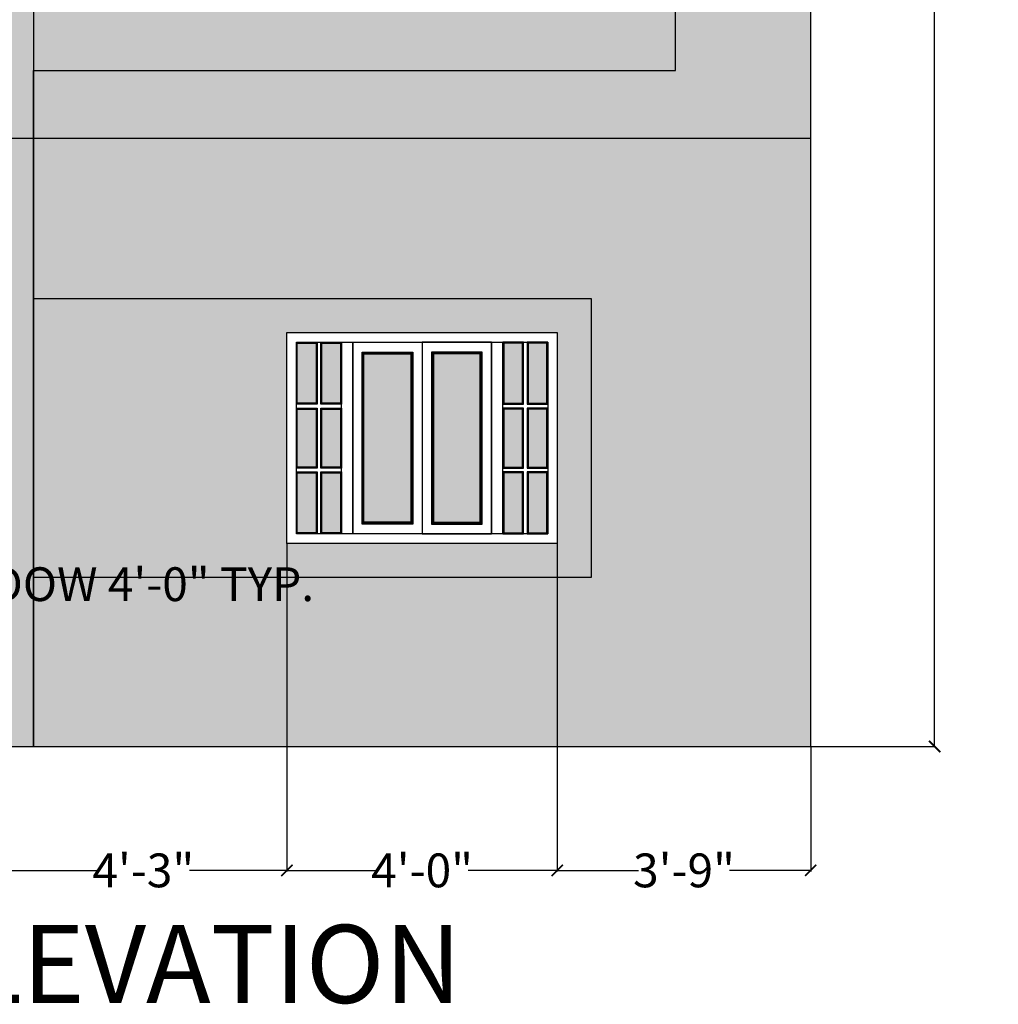
# Model space of a CAD drawing. Units: inches. Extents: x 528 to 2620, y -1066 to 798.
# Tile 39 of 41: x 2446 to 2620, y -1066 to -891. Entities that reach past the tile are written whole.
import ezdxf

# ---------------------------------------------------------------- set-up
doc = ezdxf.new("R2010")
doc.units = ezdxf.units.IN
doc.header["$MEASUREMENT"] = 0
for name, color, linetype, lineweight in [('A-ANNO-DIMS', 2, 'Continuous', 18), ('A-ANNO-TEXT', 7, 'Continuous', 25), ('A-ELEV', 7, 'Continuous', 25), ('A-ELEV-PATT', 8, 'Continuous', 13)]:
    doc.layers.add(name, color=color, linetype=linetype, lineweight=lineweight)
doc.styles.get("Standard").update_dxf_attribs({"font": 'arial.ttf'})
doc.dimstyles.get("Standard").update_dxf_attribs({"dimtxt": 6, "dimasz": 2, "dimexe": 0.18, "dimexo": 0.0625, "dimgap": 0.09, "dimtad": 0, "dimtih": 1, "dimtoh": 1, "dimdec": 1, "dimzin": 0, "dimdsep": 46, "dimlunit": 3, "dimtxsty": 'Standard', "dimblk": 'ARCHTICK', "dimcen": 0.09, "dimadec": 0, "dimazin": 0, "dimtfac": 1, "dimtdec": 1, "dimtofl": 0, "dimtmove": 0, "dimatfit": 3, "dimfxl": 1, "dimtolj": 1, "dimtzin": 0, "dimarcsym": 0})

# ---------------------------------------------------------------- blocks, each defined once
blk = doc.blocks.new('ww')
at = {"color": 0, "linetype": 'ByBlock'}
for p, q in [((30.67, -16.13), (126.65, -16.13)), ((30.67, -91.08), (30.67, -16.13)), ((126.65, -16.13), (126.65, -91.08)), ((34.01, -19.6), (123.32, -19.6)), ((34.01, -87.61), (34.01, -19.6)), ((34.01, -19.6), (49.87, -19.6)), ((34.01, -87.61), (34.01, -19.6)), ((50.03, -87.61), (50.03, -19.6)), ((54.03, -19.6), (54.03, -87.61)), ((103.29, -19.6), (103.29, -87.61)), ((107.29, -87.61), (107.29, -19.6)), ((123.32, -19.6), (123.32, -87.61)), ((123.32, -87.61), (34.01, -87.61)), ((126.65, -91.08), (30.67, -91.08))]:
    blk.add_line(p, q, dxfattribs=at)
at = {"color": 0, "linetype": 'ByBlock', "ltscale": 25}
for p, q in [((34.01, -41.58), (34.01, -19.6)), ((34.01, -19.6), (41.35, -19.6)), ((34.34, -41.23), (34.34, -19.95)), ((34.34, -19.95), (41.02, -19.95)), ((41.02, -19.95), (41.02, -41.23)), ((41.35, -19.6), (41.35, -41.58)), ((42.69, -41.58), (42.69, -19.6)), ((42.69, -19.6), (50.03, -19.6)), ((43.02, -41.23), (43.02, -19.95)), ((43.02, -19.95), (49.7, -19.95)), ((49.7, -19.95), (49.7, -41.23)), ((50.03, -19.6), (50.03, -41.58)), ((54.03, -87.61), (54.03, -19.6)), ((54.03, -19.6), (78.66, -19.6)), ((103.29, -19.6), (78.66, -19.6)), ((78.66, -19.6), (78.66, -87.61)), ((78.66, -19.6), (78.66, -87.61)), ((103.29, -87.61), (103.29, -19.6)), ((107.29, -19.6), (107.29, -41.58)), ((114.63, -19.6), (107.29, -19.6)), ((107.62, -19.95), (107.62, -41.23)), ((114.3, -19.95), (107.62, -19.95)), ((114.3, -41.23), (114.3, -19.95)), ((114.63, -41.58), (114.63, -19.6)), ((115.97, -19.6), (115.97, -41.58)), ((123.32, -19.6), (115.97, -19.6)), ((116.3, -19.95), (116.3, -41.23)), ((122.98, -19.95), (116.3, -19.95)), ((122.98, -41.23), (122.98, -19.95)), ((123.32, -41.58), (123.32, -19.6)), ((57.37, -84.14), (57.37, -23.07)), ((57.37, -23.07), (75.33, -23.07)), ((57.7, -83.8), (57.7, -23.42)), ((57.7, -23.42), (74.99, -23.42)), ((58.03, -83.45), (58.03, -23.77)), ((58.03, -23.77), (74.66, -23.77)), ((74.66, -23.77), (74.66, -83.45)), ((74.99, -23.42), (74.99, -83.8)), ((75.33, -23.07), (75.33, -84.14)), ((99.96, -23.07), (81.99, -23.07)), ((81.99, -23.07), (81.99, -84.14)), ((99.62, -23.42), (82.33, -23.42)), ((82.33, -23.42), (82.33, -83.8)), ((99.29, -23.77), (82.66, -23.77)), ((82.66, -23.77), (82.66, -83.45)), ((99.29, -83.45), (99.29, -23.77)), ((99.62, -83.8), (99.62, -23.42)), ((99.96, -84.14), (99.96, -23.07)), ((41.35, -41.58), (34.01, -41.58)), ((41.02, -41.23), (34.34, -41.23)), ((50.03, -41.58), (42.69, -41.58)), ((49.7, -41.23), (43.02, -41.23)), ((107.29, -41.58), (114.63, -41.58)), ((107.62, -41.23), (114.3, -41.23)), ((115.97, -41.58), (123.32, -41.58)), ((116.3, -41.23), (122.98, -41.23)), ((34.01, -64.25), (34.01, -42.97)), ((34.01, -42.97), (41.35, -42.97)), ((34.34, -63.9), (34.34, -43.31)), ((34.34, -43.31), (41.02, -43.31)), ((41.02, -43.31), (41.02, -63.9)), ((41.35, -42.97), (41.35, -64.25)), ((42.69, -64.25), (42.69, -42.97)), ((42.69, -42.97), (50.03, -42.97)), ((43.02, -63.9), (43.02, -43.31)), ((43.02, -43.31), (49.7, -43.31)), ((49.7, -43.31), (49.7, -63.9)), ((50.03, -42.97), (50.03, -64.25)), ((107.29, -42.97), (107.29, -64.25)), ((114.63, -42.97), (107.29, -42.97)), ((107.62, -43.31), (107.62, -63.9)), ((114.3, -43.31), (107.62, -43.31)), ((114.3, -63.9), (114.3, -43.31)), ((114.63, -64.25), (114.63, -42.97)), ((115.97, -42.97), (115.97, -64.25)), ((123.32, -42.97), (115.97, -42.97)), ((116.3, -43.31), (116.3, -63.9)), ((122.98, -43.31), (116.3, -43.31)), ((122.98, -63.9), (122.98, -43.31)), ((123.32, -64.25), (123.32, -42.97)), ((41.35, -64.25), (34.01, -64.25)), ((34.01, -87.61), (34.01, -65.64)), ((34.01, -65.64), (41.35, -65.64)), ((41.02, -63.9), (34.34, -63.9)), ((34.34, -87.27), (34.34, -65.98)), ((34.34, -65.98), (41.02, -65.98)), ((41.02, -65.98), (41.02, -87.27)), ((41.35, -65.64), (41.35, -87.61)), ((50.03, -64.25), (42.69, -64.25)), ((42.69, -87.61), (42.69, -65.64)), ((42.69, -65.64), (50.03, -65.64)), ((49.7, -63.9), (43.02, -63.9)), ((43.02, -87.27), (43.02, -65.98)), ((43.02, -65.98), (49.7, -65.98)), ((49.7, -65.98), (49.7, -87.27)), ((50.03, -65.64), (50.03, -87.61)), ((107.29, -64.25), (114.63, -64.25)), ((107.29, -65.64), (107.29, -87.61)), ((114.63, -65.64), (107.29, -65.64)), ((107.62, -63.9), (114.3, -63.9)), ((107.62, -65.98), (107.62, -87.27)), ((114.3, -65.98), (107.62, -65.98)), ((114.3, -87.27), (114.3, -65.98)), ((114.63, -87.61), (114.63, -65.64)), ((115.97, -64.25), (123.32, -64.25)), ((115.97, -65.64), (115.97, -87.61)), ((123.32, -65.64), (115.97, -65.64)), ((116.3, -63.9), (122.98, -63.9)), ((116.3, -65.98), (116.3, -87.27)), ((122.98, -65.98), (116.3, -65.98)), ((122.98, -87.27), (122.98, -65.98)), ((123.32, -87.61), (123.32, -65.64)), ((74.99, -83.8), (57.7, -83.8)), ((74.66, -83.45), (58.03, -83.45)), ((82.33, -83.8), (99.62, -83.8)), ((82.66, -83.45), (99.29, -83.45)), ((41.02, -87.27), (34.34, -87.27)), ((49.7, -87.27), (43.02, -87.27)), ((75.33, -84.14), (57.37, -84.14)), ((81.99, -84.14), (99.96, -84.14)), ((107.62, -87.27), (114.3, -87.27)), ((116.3, -87.27), (122.98, -87.27)), ((41.35, -87.61), (34.01, -87.61)), ((50.03, -87.61), (42.69, -87.61)), ((78.66, -87.61), (54.03, -87.61)), ((78.66, -87.61), (103.29, -87.61)), ((107.29, -87.61), (114.63, -87.61)), ((115.97, -87.61), (123.32, -87.61))]:
    blk.add_line(p, q, dxfattribs=at)
blk = doc.blocks.new('_ArchTick')
at = {"color": 0, "linetype": 'ByBlock', "const_width": 0.15}
blk.add_lwpolyline([(-0.5, -0.5), (0.5, 0.5)], dxfattribs=at)
blk = doc.blocks.new('*D54')
at = {"layer": 'A-ANNO-DIMS', "color": 0, "lineweight": -2, "transparency": 16777216}
for p, q in [((2327.05, -984.21), (2327.05, -991.53)), ((2375.05, -984.21), (2375.05, -991.53)), ((2327.05, -991.35), (2375.05, -991.35)), ((2375.05, -991.35), (2377.05, -991.35))]:
    blk.add_line(p, q, dxfattribs=at)
at = {"layer": 'Defpoints', "color": 0, "transparency": 16777216}
for p in [(2327.05, -984.15), (2375.05, -984.15), (2375.05, -991.35)]:
    blk.add_point(p, dxfattribs=at)
at = {"layer": 'A-ANNO-DIMS', "color": 0, "lineweight": -2, "transparency": 16777216, "xscale": 2, "yscale": 2, "zscale": 2, "rotation": 180}
blk.add_blockref('_ArchTick', (2327.05, -991.35), dxfattribs=at)
at = {"layer": 'A-ANNO-DIMS', "color": 0, "lineweight": -2, "transparency": 16777216, "xscale": 2, "yscale": 2, "zscale": 2}
blk.add_blockref('_ArchTick', (2375.05, -991.35), dxfattribs=at)
at = {"layer": 'A-ANNO-DIMS', "color": 0, "transparency": 16777216, "insert": (2439.5, -991.35), "char_height": 6, "attachment_point": 5}
blk.add_mtext('\\A1;ELEVATION WINDOW 4\'-0" TYP.', dxfattribs=at)
blk = doc.blocks.new('*D69')
at = {"layer": 'A-ANNO-DIMS', "color": 0, "lineweight": -2, "transparency": 16777216}
for p, q in [((2586.61, -660.15), (2608.73, -660.15)), ((2608.55, -660.15), (2608.55, -836.99)), ((2608.55, -1020.15), (2608.55, -843.3)), ((2586.61, -1020.15), (2608.73, -1020.15))]:
    blk.add_line(p, q, dxfattribs=at)
at = {"layer": 'Defpoints', "color": 0, "transparency": 16777216}
for p in [(2586.55, -660.15), (2608.55, -660.15), (2586.55, -1020.15)]:
    blk.add_point(p, dxfattribs=at)
at = {"layer": 'A-ANNO-DIMS', "color": 0, "lineweight": -2, "transparency": 16777216, "xscale": 2, "yscale": 2, "zscale": 2}
for p, rotation in [((2608.55, -660.15), 90), ((2608.55, -1020.15), 270)]:
    blk.add_blockref('_ArchTick', p, dxfattribs=dict(at, rotation=rotation))
at = {"layer": 'A-ANNO-DIMS', "color": 0, "transparency": 16777216, "insert": (2608.55, -840.15), "char_height": 6, "attachment_point": 5}
blk.add_mtext('\\A1;30\'-0"', dxfattribs=at)
blk = doc.blocks.new('*D85')
at = {"layer": 'A-ANNO-DIMS', "color": 0, "lineweight": -2, "transparency": 16777216}
for p, q in [((2493.55, -984.21), (2493.55, -1042.33)), ((2442.55, -1020.21), (2442.55, -1042.33)), ((2442.55, -1042.15), (2459.86, -1042.15)), ((2493.55, -1042.15), (2476.23, -1042.15))]:
    blk.add_line(p, q, dxfattribs=at)
at = {"layer": 'Defpoints', "color": 0, "transparency": 16777216}
for p in [(2493.55, -984.15), (2442.55, -1020.15), (2493.55, -1042.15)]:
    blk.add_point(p, dxfattribs=at)
at = {"layer": 'A-ANNO-DIMS', "color": 0, "lineweight": -2, "transparency": 16777216, "xscale": 2, "yscale": 2, "zscale": 2, "rotation": 180}
blk.add_blockref('_ArchTick', (2442.55, -1042.15), dxfattribs=at)
at = {"layer": 'A-ANNO-DIMS', "color": 0, "lineweight": -2, "transparency": 16777216, "xscale": 2, "yscale": 2, "zscale": 2}
blk.add_blockref('_ArchTick', (2493.55, -1042.15), dxfattribs=at)
at = {"layer": 'A-ANNO-DIMS', "color": 0, "transparency": 16777216, "insert": (2468.05, -1042.15), "char_height": 6, "attachment_point": 5}
blk.add_mtext('\\A1;4\'-3"', dxfattribs=at)
blk = doc.blocks.new('*D86')
at = {"layer": 'A-ANNO-DIMS', "color": 0, "lineweight": -2, "transparency": 16777216}
for p, q in [((2493.55, -984.21), (2493.55, -1042.33)), ((2541.55, -984.21), (2541.55, -1042.33)), ((2493.55, -1042.15), (2509.36, -1042.15)), ((2541.55, -1042.15), (2525.73, -1042.15))]:
    blk.add_line(p, q, dxfattribs=at)
at = {"layer": 'Defpoints', "color": 0, "transparency": 16777216}
for p in [(2493.55, -984.15), (2541.55, -984.15), (2541.55, -1042.15)]:
    blk.add_point(p, dxfattribs=at)
at = {"layer": 'A-ANNO-DIMS', "color": 0, "lineweight": -2, "transparency": 16777216, "xscale": 2, "yscale": 2, "zscale": 2, "rotation": 180}
blk.add_blockref('_ArchTick', (2493.55, -1042.15), dxfattribs=at)
at = {"layer": 'A-ANNO-DIMS', "color": 0, "lineweight": -2, "transparency": 16777216, "xscale": 2, "yscale": 2, "zscale": 2}
blk.add_blockref('_ArchTick', (2541.55, -1042.15), dxfattribs=at)
at = {"layer": 'A-ANNO-DIMS', "color": 0, "transparency": 16777216, "insert": (2517.55, -1042.15), "char_height": 6, "attachment_point": 5}
blk.add_mtext('\\A1;4\'-0"', dxfattribs=at)
blk = doc.blocks.new('*D87')
at = {"layer": 'A-ANNO-DIMS', "color": 0, "lineweight": -2, "transparency": 16777216}
for p, q in [((2541.55, -984.21), (2541.55, -1042.33)), ((2586.55, -1020.21), (2586.55, -1042.33)), ((2541.55, -1042.15), (2555.98, -1042.15)), ((2586.55, -1042.15), (2572.11, -1042.15))]:
    blk.add_line(p, q, dxfattribs=at)
at = {"layer": 'Defpoints', "color": 0, "transparency": 16777216}
for p in [(2541.55, -984.15), (2586.55, -1020.15), (2586.55, -1042.15)]:
    blk.add_point(p, dxfattribs=at)
at = {"layer": 'A-ANNO-DIMS', "color": 0, "lineweight": -2, "transparency": 16777216, "xscale": 2, "yscale": 2, "zscale": 2, "rotation": 180}
blk.add_blockref('_ArchTick', (2541.55, -1042.15), dxfattribs=at)
at = {"layer": 'A-ANNO-DIMS', "color": 0, "lineweight": -2, "transparency": 16777216, "xscale": 2, "yscale": 2, "zscale": 2}
blk.add_blockref('_ArchTick', (2586.55, -1042.15), dxfattribs=at)
at = {"layer": 'A-ANNO-DIMS', "color": 0, "transparency": 16777216, "insert": (2564.05, -1042.15), "char_height": 6, "attachment_point": 5}
blk.add_mtext('\\A1;3\'-9"', dxfattribs=at)

msp = doc.modelspace()

# ---------------------------------------------------------------- hatches: boundary and pattern name
at = {"layer": 'A-ELEV-PATT', "transparency": 33554687}
h = msp.add_hatch(color=256, dxfattribs=at)
h.dxf.hatch_style = 1
h.paths.add_polyline_path([(2586.55, -660.15), (2298.55, -660.15), (2298.55, -720.15), (2310.55, -720.15), (2310.55, -672.15), (2562.55, -672.15), (2562.55, -900.15), (2448.55, -900.15), (2448.55, -912.15), (2586.55, -912.15)])
h = msp.add_hatch(color=256, dxfattribs=at)
h.dxf.hatch_style = 1
h.paths.add_polyline_path([(2448.55, -756.15), (2270.55, -756.15), (2270.55, -780.15), (2436.55, -780.15), (2436.55, -888.15), (2266.05, -888.15), (2266.05, -912.15), (2448.55, -912.15)])
h = msp.add_hatch(color=256, dxfattribs=at)
h.dxf.hatch_style = 1
h.paths.add_polyline_path([(2586.55, -912.15), (2448.55, -912.15), (2448.55, -940.66), (2547.55, -940.66), (2547.55, -990.15), (2448.55, -990.15), (2448.55, -1020.15), (2586.55, -1020.15)])
h.paths.add_polyline_path([(2481.55, -789.84), (2562.55, -789.84), (2562.55, -761.55), (2448.55, -761.55), (2448.55, -900.15), (2562.55, -900.15), (2562.55, -876.97), (2481.55, -876.97), (2481.55, -833.41)])
h.paths.add_polyline_path([(2412.55, -780.15), (2298.55, -780.15), (2298.55, -852.15), (2322.55, -852.15), (2322.55, -814.66), (2370.55, -814.66), (2370.55, -852.15), (2412.55, -852.15)])
h.paths.add_polyline_path([(2394.55, -940.36), (2442.55, -940.36), (2442.55, -1020.15), (2448.55, -1020.15), (2448.55, -990.15), (2448.55, -912.15), (2310.55, -912.15), (2310.55, -1020.15), (2394.55, -1020.15)])
h.paths.add_polyline_path([(2327.05, -984.15), (2327.05, -946.66), (2375.05, -946.66), (2375.05, -984.15)], flags=16)
h.paths.add_polyline_path([(2328.71, -982.41), (2328.71, -948.4), (2336.65, -948.4), (2336.73, -948.4), (2373.38, -948.4), (2373.38, -982.41), (2369.7, -982.41)], flags=0)
h.paths.add_polyline_path([(2338.73, -982.41), (2338.73, -948.4), (2351.05, -948.4), (2363.36, -948.4), (2363.36, -982.41), (2351.05, -982.41)], flags=0)
h.paths.add_polyline_path([(2340.4, -980.68), (2340.4, -950.13), (2349.38, -950.13), (2349.38, -980.68)], flags=0)
h.paths.add_polyline_path([(2340.73, -980.33), (2340.73, -950.48), (2349.05, -950.48), (2349.05, -980.33)], flags=0)
h.paths.add_polyline_path([(2352.71, -980.68), (2352.71, -950.13), (2361.7, -950.13), (2361.7, -980.68)], flags=0)
h.paths.add_polyline_path([(2353.05, -980.33), (2353.05, -950.48), (2361.36, -950.48), (2361.36, -980.33)], flags=0)
h.paths.add_polyline_path([(2336.73, -982.41), (2333.05, -982.41), (2333.05, -971.42), (2336.73, -971.42), (2336.73, -970.73), (2333.05, -970.73), (2333.05, -960.08), (2336.73, -960.08), (2336.73, -959.39), (2333.05, -959.39), (2333.05, -948.57), (2336.73, -948.57)], flags=0)
h.paths.add_polyline_path([(2333.22, -982.24), (2333.22, -971.6), (2336.73, -971.6), (2336.73, -982.24)], flags=0)
h.paths.add_polyline_path([(2332.39, -982.41), (2328.71, -982.41), (2328.71, -948.4), (2332.39, -948.4), (2332.39, -959.39), (2328.71, -959.39), (2328.71, -960.08), (2332.39, -960.08), (2332.39, -970.73), (2328.71, -970.73), (2328.71, -971.42), (2332.39, -971.42)], flags=0)
h.paths.add_polyline_path([(2332.22, -982.24), (2328.71, -982.24), (2328.71, -971.6), (2332.22, -971.6)], flags=0)
h.paths.add_polyline_path([(2365.36, -982.41), (2365.36, -948.4), (2369.04, -948.4), (2369.04, -959.39), (2365.36, -959.39), (2365.36, -960.08), (2369.04, -960.08), (2369.04, -970.73), (2365.36, -970.73), (2365.36, -971.42), (2369.04, -971.42), (2369.04, -982.41)], flags=0)
h.paths.add_polyline_path([(2369.7, -971.42), (2373.38, -971.42), (2373.38, -982.24), (2369.7, -982.24)], flags=0)
h.paths.add_polyline_path([(2333.22, -970.55), (2333.22, -960.26), (2336.73, -960.26), (2336.73, -970.55)], flags=0)
h.paths.add_polyline_path([(2332.22, -970.55), (2328.71, -970.55), (2328.71, -960.26), (2332.22, -960.26)], flags=0)
h.paths.add_polyline_path([(2369.7, -970.73), (2369.7, -960.08), (2373.38, -960.08), (2373.38, -970.73)], flags=0)
h.paths.add_polyline_path([(2336.56, -959.22), (2336.56, -948.57), (2336.73, -948.4), (2336.73, -959.22)], flags=0)
h.paths.add_polyline_path([(2332.22, -959.22), (2328.71, -959.22), (2328.71, -948.57), (2332.22, -948.57)], flags=0)
h.paths.add_polyline_path([(2369.7, -959.39), (2369.7, -948.4), (2373.38, -948.4), (2373.38, -959.39)], flags=0)
h = msp.add_hatch(color=256, dxfattribs=at)
h.dxf.hatch_style = 1
h.paths.add_polyline_path([(2562.55, -789.84), (2481.55, -789.84), (2481.55, -833.41), (2481.55, -876.97), (2562.55, -876.97)])
h.paths.add_polyline_path([(2541.55, -852.15), (2493.55, -852.15), (2493.55, -814.66), (2487.57, -814.66), (2487.57, -808.71), (2546.5, -808.65), (2546.5, -814.66), (2541.55, -814.66)], flags=16)
h.paths.add_polyline_path([(2539.88, -850.41), (2536.2, -850.41), (2495.21, -850.41), (2495.21, -816.4), (2503.15, -816.4), (2503.23, -816.4), (2539.88, -816.4)], flags=0)
h.paths.add_polyline_path([(2539.88, -838.73), (2536.2, -838.73), (2536.2, -828.08), (2539.88, -828.08)], flags=0)
h.paths.add_polyline_path([(2539.88, -839.42), (2539.88, -850.24), (2536.2, -850.24), (2536.2, -839.42)], flags=0)
h.paths.add_polyline_path([(2539.71, -838.55), (2536.37, -838.55), (2536.37, -828.26), (2539.71, -828.26)], flags=0)
h.paths.add_polyline_path([(2535.54, -838.73), (2531.86, -838.73), (2531.86, -839.42), (2535.54, -839.42), (2535.54, -850.41), (2531.86, -850.41), (2531.86, -816.4), (2535.54, -816.4), (2535.54, -827.39), (2531.86, -827.39), (2531.86, -828.08), (2535.54, -828.08)], flags=0)
h.paths.add_polyline_path([(2535.37, -838.55), (2531.86, -838.55), (2531.86, -828.26), (2535.37, -828.26)], flags=0)
h.paths.add_polyline_path([(2535.37, -839.6), (2535.37, -850.24), (2531.86, -850.24), (2531.86, -839.6)], flags=0)
h.paths.add_polyline_path([(2539.88, -827.39), (2536.2, -827.39), (2536.2, -816.4), (2539.88, -816.4)], flags=0)
h.paths.add_polyline_path([(2539.71, -827.22), (2536.37, -827.22), (2536.37, -816.57), (2539.71, -816.57)], flags=0)
h.paths.add_polyline_path([(2535.37, -827.22), (2531.86, -827.22), (2531.86, -816.57), (2535.37, -816.57)], flags=0)
h.paths.add_polyline_path([(2529.86, -850.41), (2517.55, -850.41), (2505.23, -850.41), (2505.23, -816.4), (2517.55, -816.4), (2529.86, -816.4)], flags=0)
h.paths.add_polyline_path([(2528.2, -848.68), (2519.21, -848.68), (2519.21, -818.13), (2528.2, -818.13)], flags=0)
h.paths.add_polyline_path([(2528.03, -848.5), (2519.38, -848.5), (2519.38, -818.31), (2528.03, -818.31)], flags=0)
h.paths.add_polyline_path([(2527.86, -848.33), (2519.55, -848.33), (2519.55, -818.48), (2527.86, -818.48)], flags=0)
h.paths.add_polyline_path([(2515.88, -848.68), (2506.9, -848.68), (2506.9, -818.13), (2515.88, -818.13)], flags=0)
h.paths.add_polyline_path([(2515.71, -848.5), (2507.06, -848.5), (2507.06, -818.31), (2515.71, -818.31)], flags=0)
h.paths.add_polyline_path([(2515.55, -848.33), (2507.23, -848.33), (2507.23, -818.48), (2515.55, -818.48)], flags=0)
h.paths.add_polyline_path([(2503.23, -850.41), (2499.55, -850.41), (2499.55, -839.42), (2503.23, -839.42), (2503.23, -838.73), (2499.55, -838.73), (2499.55, -828.08), (2503.23, -828.08), (2503.23, -827.39), (2499.55, -827.39), (2499.55, -816.57), (2503.23, -816.57)], flags=0)
h.paths.add_polyline_path([(2503.23, -838.55), (2499.72, -838.55), (2499.72, -828.26), (2503.23, -828.26)], flags=0)
h.paths.add_polyline_path([(2503.23, -850.24), (2499.72, -850.24), (2499.72, -839.6), (2503.23, -839.6)], flags=0)
h.paths.add_polyline_path([(2503.06, -816.57), (2503.23, -816.4), (2503.23, -827.22), (2503.06, -827.22)], flags=0)
h.paths.add_polyline_path([(2498.89, -838.73), (2495.21, -838.73), (2495.21, -839.42), (2498.89, -839.42), (2498.89, -850.41), (2495.21, -850.41), (2495.21, -816.4), (2498.89, -816.4), (2498.89, -827.39), (2495.21, -827.39), (2495.21, -828.08), (2498.89, -828.08)], flags=0)
h.paths.add_polyline_path([(2498.72, -838.55), (2495.21, -838.55), (2495.21, -828.26), (2498.72, -828.26)], flags=0)
h.paths.add_polyline_path([(2498.72, -839.6), (2498.72, -850.24), (2495.21, -850.24), (2495.21, -839.6)], flags=0)
h.paths.add_polyline_path([(2498.72, -827.22), (2495.21, -827.22), (2495.21, -816.57), (2498.72, -816.57)], flags=0)
h.paths.add_polyline_path([(2547.55, -940.66), (2448.55, -940.66), (2448.55, -990.15), (2547.55, -990.15)])
h.paths.add_polyline_path([(2493.55, -946.66), (2541.55, -946.66), (2541.55, -984.15), (2493.55, -984.15)], flags=16)
h.paths.add_polyline_path([(2495.21, -948.4), (2503.15, -948.4), (2503.23, -948.4), (2539.88, -948.4), (2539.88, -982.41), (2536.2, -982.41), (2495.21, -982.41)], flags=0)
h.paths.add_polyline_path([(2495.21, -948.4), (2498.89, -948.4), (2498.89, -959.39), (2495.21, -959.39), (2495.21, -960.08), (2498.89, -960.08), (2498.89, -970.73), (2495.21, -970.73), (2495.21, -971.42), (2498.89, -971.42), (2498.89, -982.41), (2495.21, -982.41)], flags=0)
h.paths.add_polyline_path([(2498.72, -960.26), (2498.72, -970.55), (2495.21, -970.55), (2495.21, -960.26)], flags=0)
h.paths.add_polyline_path([(2498.72, -971.6), (2498.72, -982.24), (2495.21, -982.24), (2495.21, -971.6)], flags=0)
h.paths.add_polyline_path([(2499.55, -948.57), (2503.23, -948.57), (2503.23, -982.41), (2499.55, -982.41), (2499.55, -971.42), (2503.23, -971.42), (2503.23, -970.73), (2499.55, -970.73), (2499.55, -960.08), (2503.23, -960.08), (2503.23, -959.39), (2499.55, -959.39)], flags=0)
h.paths.add_polyline_path([(2503.06, -959.22), (2503.06, -948.57), (2503.23, -948.4), (2503.23, -959.22)], flags=0)
h.paths.add_polyline_path([(2499.72, -960.26), (2503.23, -960.26), (2503.23, -970.55), (2499.72, -970.55)], flags=0)
h.paths.add_polyline_path([(2499.72, -971.6), (2503.23, -971.6), (2503.23, -982.24), (2499.72, -982.24)], flags=0)
h.paths.add_polyline_path([(2505.23, -948.4), (2517.55, -948.4), (2529.86, -948.4), (2529.86, -982.41), (2517.55, -982.41), (2505.23, -982.41)], flags=0)
h.paths.add_polyline_path([(2506.9, -950.13), (2515.88, -950.13), (2515.88, -980.68), (2506.9, -980.68)], flags=0)
h.paths.add_polyline_path([(2507.23, -950.48), (2515.55, -950.48), (2515.55, -980.33), (2507.23, -980.33)], flags=0)
h.paths.add_polyline_path([(2519.21, -950.13), (2528.2, -950.13), (2528.2, -980.68), (2519.21, -980.68)], flags=0)
h.paths.add_polyline_path([(2519.55, -950.48), (2527.86, -950.48), (2527.86, -980.33), (2519.55, -980.33)], flags=0)
h.paths.add_polyline_path([(2531.86, -948.4), (2535.54, -948.4), (2535.54, -959.39), (2531.86, -959.39), (2531.86, -960.08), (2535.54, -960.08), (2535.54, -970.73), (2531.86, -970.73), (2531.86, -971.42), (2535.54, -971.42), (2535.54, -982.41), (2531.86, -982.41)], flags=0)
h.paths.add_polyline_path([(2535.37, -960.26), (2535.37, -970.55), (2531.86, -970.55), (2531.86, -960.26)], flags=0)
h.paths.add_polyline_path([(2535.37, -971.6), (2535.37, -982.24), (2531.86, -982.24), (2531.86, -971.6)], flags=0)
h.paths.add_polyline_path([(2536.2, -948.4), (2539.88, -948.4), (2539.88, -959.39), (2536.2, -959.39)], flags=0)
h.paths.add_polyline_path([(2536.2, -960.08), (2539.88, -960.08), (2539.88, -970.73), (2536.2, -970.73)], flags=0)
h.paths.add_polyline_path([(2536.2, -971.42), (2539.88, -971.42), (2539.88, -982.24), (2536.2, -982.24)], flags=0)
h = msp.add_hatch(color=256, dxfattribs=at)
h.dxf.hatch_style = 1
h.paths.add_polyline_path([(2527.86, -818.48), (2519.55, -818.48), (2519.55, -848.33), (2527.86, -848.33)])
h.paths.add_polyline_path([(2515.55, -818.48), (2507.23, -818.48), (2507.23, -848.33), (2515.55, -848.33)])
h.paths.add_polyline_path([(2498.72, -816.57), (2495.38, -816.57), (2495.38, -827.22), (2498.72, -827.22)])
h.paths.add_polyline_path([(2503.06, -816.57), (2499.72, -816.57), (2499.72, -827.22), (2503.06, -827.22)])
h.paths.add_polyline_path([(2498.72, -828.26), (2495.38, -828.26), (2495.38, -838.55), (2498.72, -838.55)])
h.paths.add_polyline_path([(2503.06, -828.26), (2499.72, -828.26), (2499.72, -838.55), (2503.06, -838.55)])
h.paths.add_polyline_path([(2498.72, -839.6), (2495.38, -839.6), (2495.38, -850.24), (2498.72, -850.24)])
h.paths.add_polyline_path([(2503.06, -839.6), (2499.72, -839.6), (2499.72, -850.24), (2503.06, -850.24)])
h.paths.add_polyline_path([(2535.37, -839.6), (2532.03, -839.6), (2532.03, -850.24), (2535.37, -850.24)])
h.paths.add_polyline_path([(2539.71, -839.6), (2536.37, -839.6), (2536.37, -850.24), (2539.71, -850.24)])
h.paths.add_polyline_path([(2535.37, -828.26), (2532.03, -828.26), (2532.03, -838.55), (2535.37, -838.55)])
h.paths.add_polyline_path([(2539.71, -828.26), (2536.37, -828.26), (2536.37, -838.55), (2539.71, -838.55)])
h.paths.add_polyline_path([(2535.37, -816.57), (2532.03, -816.57), (2532.03, -827.22), (2535.37, -827.22)])
h.paths.add_polyline_path([(2356.86, -818.48), (2348.55, -818.48), (2348.55, -848.33), (2356.86, -848.33)])
h.paths.add_polyline_path([(2344.55, -818.48), (2336.23, -818.48), (2336.23, -848.33), (2344.55, -848.33)])
h.paths.add_polyline_path([(2327.72, -816.57), (2324.38, -816.57), (2324.38, -827.22), (2327.72, -827.22)])
h.paths.add_polyline_path([(2332.06, -816.57), (2328.72, -816.57), (2328.72, -827.22), (2332.06, -827.22)])
h.paths.add_polyline_path([(2327.72, -828.26), (2324.38, -828.26), (2324.38, -838.55), (2327.72, -838.55)])
h.paths.add_polyline_path([(2332.06, -828.26), (2328.72, -828.26), (2328.72, -838.55), (2332.06, -838.55)])
h.paths.add_polyline_path([(2327.72, -839.6), (2324.38, -839.6), (2324.38, -850.24), (2327.72, -850.24)])
h.paths.add_polyline_path([(2332.06, -839.6), (2328.72, -839.6), (2328.72, -850.24), (2332.06, -850.24)])
h.paths.add_polyline_path([(2368.71, -839.6), (2365.37, -839.6), (2365.37, -850.24), (2368.71, -850.24)])
h.paths.add_polyline_path([(2364.37, -839.6), (2361.03, -839.6), (2361.03, -850.24), (2364.37, -850.24)])
h.paths.add_polyline_path([(2364.37, -828.26), (2361.03, -828.26), (2361.03, -838.55), (2364.37, -838.55)])
h.paths.add_polyline_path([(2368.71, -828.26), (2365.37, -828.26), (2365.37, -838.55), (2368.71, -838.55)])
h.paths.add_polyline_path([(2364.37, -816.57), (2361.03, -816.57), (2361.03, -827.22), (2364.37, -827.22)])
h.paths.add_polyline_path([(2368.71, -816.57), (2365.37, -816.57), (2365.37, -827.22), (2368.71, -827.22)])
h.paths.add_polyline_path([(2361.36, -950.48), (2353.05, -950.48), (2353.05, -980.33), (2361.36, -980.33)])
h.paths.add_polyline_path([(2349.05, -950.48), (2340.73, -950.48), (2340.73, -980.33), (2349.05, -980.33)])
h.paths.add_polyline_path([(2336.56, -971.6), (2333.22, -971.6), (2333.22, -982.24), (2336.56, -982.24)])
h.paths.add_polyline_path([(2332.22, -971.6), (2328.88, -971.6), (2328.88, -982.24), (2332.22, -982.24)])
h.paths.add_polyline_path([(2336.56, -960.26), (2333.22, -960.26), (2333.22, -970.55), (2336.56, -970.55)])
h.paths.add_polyline_path([(2332.22, -960.26), (2328.88, -960.26), (2328.88, -970.55), (2332.22, -970.55)])
h.paths.add_polyline_path([(2332.22, -948.57), (2328.88, -948.57), (2328.88, -959.22), (2332.22, -959.22)])
h.paths.add_polyline_path([(2336.56, -948.57), (2333.22, -948.57), (2333.22, -959.22), (2336.56, -959.22)])
h.paths.add_polyline_path([(2368.87, -971.6), (2365.53, -971.6), (2365.53, -982.24), (2368.87, -982.24)])
h.paths.add_polyline_path([(2373.21, -971.6), (2369.87, -971.6), (2369.87, -982.24), (2373.21, -982.24)])
h.paths.add_polyline_path([(2373.21, -960.26), (2369.87, -960.26), (2369.87, -970.55), (2373.21, -970.55)])
h.paths.add_polyline_path([(2368.87, -960.26), (2365.53, -960.26), (2365.53, -970.55), (2368.87, -970.55)])
h.paths.add_polyline_path([(2368.87, -948.57), (2365.53, -948.57), (2365.53, -959.22), (2368.87, -959.22)])
h.paths.add_polyline_path([(2373.21, -948.57), (2369.87, -948.57), (2369.87, -959.22), (2373.21, -959.22)])
h.paths.add_polyline_path([(2527.86, -950.48), (2519.55, -950.48), (2519.55, -980.33), (2527.86, -980.33)])
h.paths.add_polyline_path([(2515.55, -950.48), (2507.23, -950.48), (2507.23, -980.33), (2515.55, -980.33)])
h.paths.add_polyline_path([(2539.71, -971.6), (2536.37, -971.6), (2536.37, -982.24), (2539.71, -982.24)])
h.paths.add_polyline_path([(2535.37, -971.6), (2532.03, -971.6), (2532.03, -982.24), (2535.37, -982.24)])
h.paths.add_polyline_path([(2535.37, -960.26), (2532.03, -960.26), (2532.03, -970.55), (2535.37, -970.55)])
h.paths.add_polyline_path([(2539.71, -960.26), (2536.37, -960.26), (2536.37, -970.55), (2539.71, -970.55)])
h.paths.add_polyline_path([(2535.37, -948.57), (2532.03, -948.57), (2532.03, -959.22), (2535.37, -959.22)])
h.paths.add_polyline_path([(2539.71, -948.57), (2536.37, -948.57), (2536.37, -959.22), (2539.71, -959.22)])
h.paths.add_polyline_path([(2498.72, -971.6), (2495.38, -971.6), (2495.38, -982.24), (2498.72, -982.24)])
h.paths.add_polyline_path([(2503.06, -971.6), (2499.72, -971.6), (2499.72, -982.24), (2503.06, -982.24)])
h.paths.add_polyline_path([(2498.72, -960.26), (2495.38, -960.26), (2495.38, -970.55), (2498.72, -970.55)])
h.paths.add_polyline_path([(2503.06, -960.26), (2499.72, -960.26), (2499.72, -970.55), (2503.06, -970.55)])
h.paths.add_polyline_path([(2498.72, -948.57), (2495.38, -948.57), (2495.38, -959.22), (2498.72, -959.22)])
h.paths.add_polyline_path([(2503.06, -948.57), (2499.72, -948.57), (2499.72, -959.22), (2503.06, -959.22)])

# ---------------------------------------------------------------- linework, layer by layer
at = {"layer": 'A-ELEV'}
for p, q in [((2586.55, -1020.15), (2586.55, -660.15)), ((2562.55, -900.15), (2562.55, -672.15)), ((2448.55, -720.15), (2448.55, -1020.15)), ((2586.55, -1020.15), (2586.55, -894.15)), ((2448.55, -1020.15), (2448.55, -900.15)), ((2448.55, -900.15), (2562.55, -900.15)), ((2266.05, -912.15), (2448.55, -912.15)), ((2448.55, -912.15), (2586.55, -912.15)), ((2448.55, -940.66), (2547.55, -940.66)), ((2547.55, -940.66), (2547.55, -990.15)), ((2547.55, -990.15), (2448.55, -990.15)), ((2298.55, -1020.15), (2586.55, -1020.15))]:
    msp.add_line(p, q, dxfattribs=at)

# ---------------------------------------------------------------- block references
at = {"layer": 'A-ELEV', "xscale": 0.5001250312578946, "yscale": 0.5001250312578946, "zscale": 0.5001250312578946}
msp.add_blockref('ww', (2478.21, -938.6), dxfattribs=at)

# ---------------------------------------------------------------- texts
at = {"layer": 'A-ANNO-TEXT'}
msp.add_text('FRONT ELEVATION', height=13.8508, dxfattribs=at).set_placement((2359.48, -1065.68))

# ---------------------------------------------------------------- dimensions: what is measured, and where the dimension line sits
at = {"layer": 'A-ANNO-DIMS'}
dim = msp.add_linear_dim(base=(2608.55, -660.15), p1=(2586.55, -1020.15), p2=(2586.55, -660.15), angle=90, dimstyle='Standard', override={"dimdec": 1, "dimlfac": 1, "dimrnd": 0, "dimzin": 1, "dimdsep": 46, "dimlunit": 4, "dimfrac": 2}, dxfattribs=at)
dim.commit()
dim.dimension.update_dxf_attribs({"geometry": '*D69', "text_midpoint": (2608.55, -840.15)})
dim = msp.add_linear_dim(base=(2375.05, -991.35), p1=(2327.05, -984.15), p2=(2375.05, -984.15), text='ELEVATION WINDOW <> TYP.', dimstyle='Standard', override={"dimdec": 1, "dimrnd": 0, "dimzin": 1, "dimlunit": 4, "dimfrac": 2}, dxfattribs=at)
dim.commit()
dim.dimension.update_dxf_attribs({"geometry": '*D54', "text_midpoint": (2439.5, -991.35)})
for base, p1, p2, picture, middle in [((2493.55, -1042.15), (2442.55, -1020.15), (2493.55, -984.15), '*D85', (2468.05, -1042.15)), ((2541.55, -1042.15), (2493.55, -984.15), (2541.55, -984.15), '*D86', (2517.55, -1042.15)), ((2586.55, -1042.15), (2541.55, -984.15), (2586.55, -1020.15), '*D87', (2564.05, -1042.15))]:
    dim = msp.add_linear_dim(base=base, p1=p1, p2=p2, dimstyle='Standard', override={"dimdec": 1, "dimlfac": 1, "dimrnd": 0, "dimzin": 1, "dimdsep": 46, "dimlunit": 4, "dimfrac": 2}, dxfattribs=at)
    dim.commit()
    dim.dimension.update_dxf_attribs({"geometry": picture, "text_midpoint": middle})

doc.saveas('drawing.dxf')
